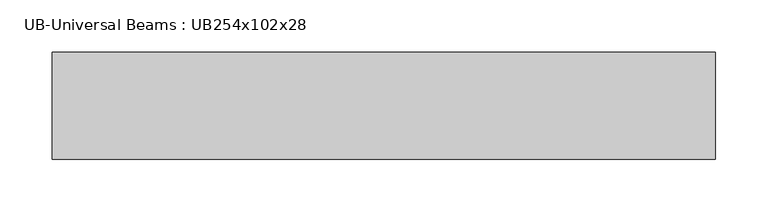
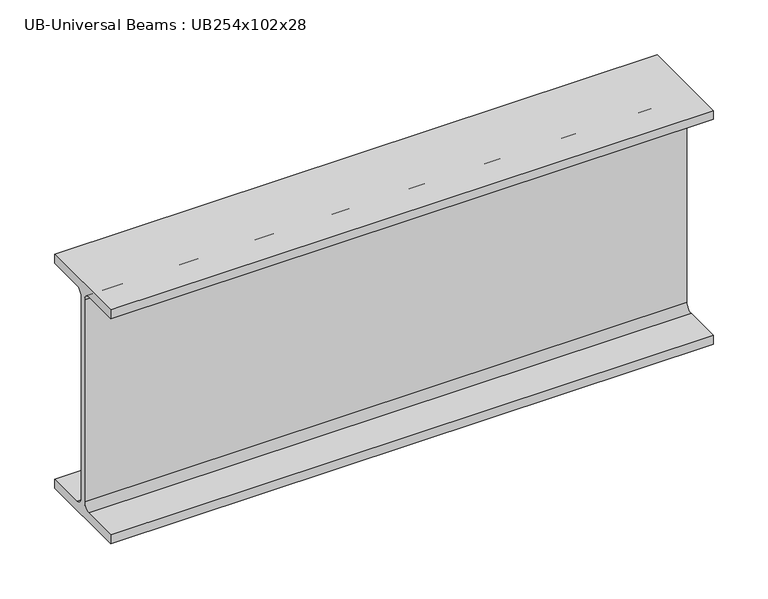
"""IFC4 building model written with IfcOpenShell, lengths in millimetres: beam geometry, UB-Universal Beams : UB254x102x28."""

from ifc_helpers import new_model, si_unit, point, frame, frame_2d, origin, place, context, project, spatial, polyline, circle_curve, trimmed, segment, composite_curve, outline, extrude, source, transform, mapped, element, save


def ub_universal_beams_ub254x102x28_9eef3cd1(model_context):
    return source(origin(), model_context, "Body", "SweptSolid", [
        extrude(outline(composite_curve([segment(polyline([(51.1, -120.2), (51.1, -130.2), (-51.1, -130.2), (-51.1, -120.2), (-10.75, -120.2)]), True, "CONTINUOUS"), segment(trimmed(circle_curve(frame_2d((-10.75, -112.6)), 7.6), [point((-10.75, -120.2))], [point((-3.15, -112.6))], True, "CARTESIAN"), True, "CONTINUOUS"), segment(polyline([(-3.15, -112.6), (-3.15, 112.6)]), True, "CONTINUOUS"), segment(trimmed(circle_curve(frame_2d((-10.75, 112.6)), 7.6), [point((-3.15, 112.6))], [point((-10.75, 120.2))], True, "CARTESIAN"), True, "CONTINUOUS"), segment(polyline([(-10.75, 120.2), (-51.1, 120.2), (-51.1, 130.2), (51.1, 130.2), (51.1, 120.2), (10.75, 120.2)]), True, "CONTINUOUS"), segment(trimmed(circle_curve(frame_2d((10.75, 112.6)), 7.6), [point((10.75, 120.2))], [point((3.15, 112.6))], True, "CARTESIAN"), True, "CONTINUOUS"), segment(polyline([(3.15, 112.6), (3.15, -112.6)]), True, "CONTINUOUS"), segment(trimmed(circle_curve(frame_2d((10.75, -112.6)), 7.6), [point((3.15, -112.6))], [point((10.75, -120.2))], True, "CARTESIAN"), True, "CONTINUOUS"), segment(polyline([(10.75, -120.2), (51.1, -120.2)]), True, "CONTINUOUS")], self_intersect=False)), frame((-365.1, 0.0, 0.0), z_axis=(1.0, 0.0, 0.0), x_axis=(0.0, 1.0, 0.0)), (0.0, 0.0, 1.0), 634.2),
    ])


if __name__ == "__main__":
    model = new_model("IFC4")
    model_context = context("Model", 3, world=origin())
    ifc_project = project(units=[si_unit("LENGTHUNIT", "METRE", prefix="MILLI")], contexts=[model_context])
    site = spatial("IfcSite", under=ifc_project)
    building = spatial("IfcBuilding", under=site)
    placement = place(None, origin())
    ub_universal_beams_ub254x102x28_shape = ub_universal_beams_ub254x102x28_9eef3cd1(model_context)
    element("IfcBeam", 1, ObjectType="UB-Universal Beams : UB254x102x28", at=placement, inside=building, context=model_context, shape_type="MappedRepresentation", body=[
        mapped(ub_universal_beams_ub254x102x28_shape, transform((0.0, 0.0, 0.0), x_axis=(1.0, 0.0, 0.0), y_axis=(0.0, 1.0, 0.0), z_axis=(0.0, 0.0, 1.0))),
    ])
    save(model, "model.ifc")

# Revit data of these elements
# Type "UB-Universal Beams : UB254x102x28"
#   Section Name Key = "UB254X102X28"
#   Width = 10.22 cm
#   Web Thickness = 0.63 cm
#   Web Fillet = 0.76 cm
#   Warping Constant = 28000.0 cm⁶
#   Torsional Moment of Inertia = 9.57 cm⁴
#   Section Area = 36.1 cm²
#   Plastic Modulus weak axis = 54.8 cm³
#   Plastic Modulus strong axis = 353.0 cm³
#   Nominal Weight = 28.2999 kgf/m
#   Moment of Inertia weak axis = 179.00 cm⁴
#   Moment of Inertia strong axis = 4005.00 cm⁴
#   Height = 26.04 cm
#   Flange Thickness = 1.0 cm
#   Elastic Modulus weak axis = 34.9 cm³
#   Elastic Modulus strong axis = 308.0 cm³
#   Centroid Vertical = 13.02 cm
#   Centroid Horizontal = 5.11 cm
#   Bolt Spacing = 5.4 cm
#   Length [instance default] = 4' - 11.05512"
#   Structural Material [instance default] = Metal - Steel 43-275
#   Type Comments = ""
#   Assembly Code = ""
# Element 1 (IfcBeam, "UB-Universal Beams : UB254x102x28")
#   Materials on its faces: "Metal - Steel 43-275"
# Materials
#   "Metal - Steel 43-275": class "Metal", colour RGB 247 247 247, transparency 0, Cost = 0
